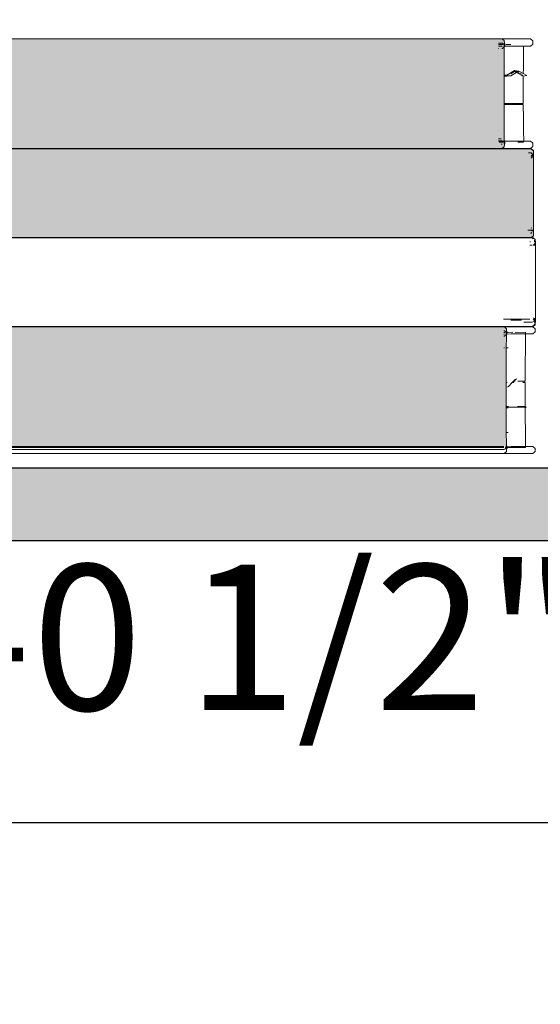
# Model space of a CAD drawing. Units: millimetres. Extents: x 7894 to 8038, y 6851 to 6951.
# Tile 18 of 49: x 7951.055 to 7954.632, y 6903.287 to 6910.053. Entities that reach past the tile are written whole.
import ezdxf

# ---------------------------------------------------------------- set-up
doc = ezdxf.new("R2010")
doc.units = ezdxf.units.MM
for name, color, linetype, lineweight in [('A-ANNO-DIMS', 2, 'Continuous', 18), ('A-FURN-BOOK', 8, 'Continuous', 13), ('A-FURN-SHLF', 7, 'Continuous', 30)]:
    doc.layers.add(name, color=color, linetype=linetype, lineweight=lineweight)
doc.layers.add('A-FURN-PATT', color=32, linetype='Continuous', lineweight=9, true_color=0xcd6928)
doc.styles.get("Standard").update_dxf_attribs({"font": 'arial.ttf'})
doc.dimstyles.new('ISO-25', dxfattribs={"dimtxt": 1, "dimasz": 1, "dimexe": 1.25, "dimexo": 0.625, "dimtad": 1, "dimdec": 0, "dimlunit": 4, "dimtxsty": 'Standard', "dimcen": 2.5, "dimclrt": 1, "dimadec": 0, "dimazin": 0, "dimtfac": 1, "dimtdec": 0, "dimtmove": 0, "dimatfit": 3, "dimfxl": 1, "dimarcsym": 0})

# ---------------------------------------------------------------- blocks, each defined once
blk = doc.blocks.new('*D23')
at = {"layer": 'A-ANNO-DIMS', "color": 0, "lineweight": -2, "transparency": 16777216}
for p, q in [((7940.0888, 6907.098), (7940.0888, 6947.7928)), ((7971.9356, 6928.989), (7971.9356, 6947.7928)), ((7941.0888, 6946.5428), (7970.9356, 6946.5428))]:
    blk.add_line(p, q, dxfattribs=at)
at = {"layer": 'A-ANNO-DIMS', "color": 0, "transparency": 16777216}
for points in [[(7941.0888, 6946.7095), (7941.0888, 6946.3762), (7940.0888, 6946.5428)], [(7970.9356, 6946.7095), (7970.9356, 6946.3762), (7971.9356, 6946.5428)]]:
    blk.add_solid(points, dxfattribs=at)
at = {"layer": 'Defpoints', "color": 0, "transparency": 16777216}
for p in [(7971.9356, 6946.5428), (7971.9356, 6928.364), (7940.0888, 6906.473)]:
    blk.add_point(p, dxfattribs=at)
at = {"layer": 'A-ANNO-DIMS', "color": 1, "transparency": 16777216, "insert": (7956.0122, 6947.6784), "char_height": 1, "attachment_point": 5}
blk.add_mtext('2\'-8"', dxfattribs=at)
blk = doc.blocks.new('*D24')
at = {"layer": 'A-ANNO-DIMS', "color": 0, "lineweight": -2, "transparency": 16777216}
for p, q in [((7953.3408, 6944.6059), (7936.9023, 6944.6059)), ((7938.1523, 6907.473), (7938.1523, 6943.6059)), ((7939.4638, 6906.473), (7936.9023, 6906.473))]:
    blk.add_line(p, q, dxfattribs=at)
at = {"layer": 'A-ANNO-DIMS', "color": 0, "transparency": 16777216}
for points in [[(7937.9856, 6943.6059), (7938.319, 6943.6059), (7938.1523, 6944.6059)], [(7937.9856, 6907.473), (7938.319, 6907.473), (7938.1523, 6906.473)]]:
    blk.add_solid(points, dxfattribs=at)
at = {"layer": 'Defpoints', "color": 0, "transparency": 16777216}
for p in [(7938.1523, 6944.6059), (7953.9658, 6944.6059), (7940.0888, 6906.473)]:
    blk.add_point(p, dxfattribs=at)
at = {"layer": 'A-ANNO-DIMS', "color": 1, "transparency": 16777216, "insert": (7937.0164, 6925.5395), "char_height": 1, "attachment_point": 5, "rotation": 90}
blk.add_mtext('3\'-2"', dxfattribs=at)
blk = doc.blocks.new('*D25')
at = {"layer": 'A-ANNO-DIMS', "color": 0, "lineweight": -2, "transparency": 16777216}
for p, q in [((7940.0888, 6905.848), (7940.0888, 6903.2865)), ((7964.3408, 6905.8484), (7964.3408, 6903.2865)), ((7941.0888, 6904.5365), (7963.3408, 6904.5365))]:
    blk.add_line(p, q, dxfattribs=at)
at = {"layer": 'A-ANNO-DIMS', "color": 0, "transparency": 16777216}
for points in [[(7941.0888, 6904.7032), (7941.0888, 6904.3699), (7940.0888, 6904.5365)], [(7963.3408, 6904.7032), (7963.3408, 6904.3699), (7964.3408, 6904.5365)]]:
    blk.add_solid(points, dxfattribs=at)
at = {"layer": 'Defpoints', "color": 0, "transparency": 16777216}
for p in [(7940.0888, 6906.473), (7964.3408, 6906.4734), (7964.3408, 6904.5365)]:
    blk.add_point(p, dxfattribs=at)
at = {"layer": 'A-ANNO-DIMS', "color": 1, "transparency": 16777216, "insert": (7952.2148, 6905.6786), "char_height": 1, "attachment_point": 5}
blk.add_mtext('2\'-0 1/2"', dxfattribs=at)
blk = doc.blocks.new('*D26')
at = {"layer": 'A-ANNO-DIMS', "color": 0, "lineweight": -2, "transparency": 16777216}
for p, q in [((7950.9654, 6918.7198), (7975.2272, 6918.7198)), ((7973.9772, 6917.7198), (7973.9772, 6907.4734)), ((7964.9658, 6906.4734), (7975.2272, 6906.4734))]:
    blk.add_line(p, q, dxfattribs=at)
at = {"layer": 'A-ANNO-DIMS', "color": 0, "transparency": 16777216}
for points in [[(7973.8105, 6917.7198), (7974.1439, 6917.7198), (7973.9772, 6918.7198)], [(7973.8105, 6907.4734), (7974.1439, 6907.4734), (7973.9772, 6906.4734)]]:
    blk.add_solid(points, dxfattribs=at)
at = {"layer": 'Defpoints', "color": 0, "transparency": 16777216}
for p in [(7950.3404, 6918.7198), (7964.3408, 6906.4734), (7973.9772, 6906.4734)]:
    blk.add_point(p, dxfattribs=at)
at = {"layer": 'A-ANNO-DIMS', "color": 1, "transparency": 16777216, "insert": (7972.8416, 6912.5966), "char_height": 1, "attachment_point": 5, "rotation": 90}
blk.add_mtext('1\'-0"', dxfattribs=at)

msp = doc.modelspace()

# ---------------------------------------------------------------- hatches: boundary and pattern name
at = {"layer": 'A-FURN-PATT'}
h = msp.add_hatch(color=256, dxfattribs=at)
h.dxf.hatch_style = 1
h.paths.add_polyline_path([(7942.8406, 6913.3629), (7942.8593, 6913.356), (7942.8677, 6913.356), (7942.8677, 6914.2132), (7942.876, 6914.2376), (7942.8813, 6914.2376), (7942.9022, 6914.2457), (7943.3657, 6914.2457), (7943.3844, 6914.2376), (7943.3861, 6914.2376), (7943.3858, 6914.2132), (7943.3852, 6913.2312), (7943.3944, 6906.9948), (7943.387, 6906.9732), (7943.4027, 6906.9732), (7943.403, 6906.9948), (7943.4029, 6908.4372), (7943.3944, 6914.2132), (7943.4169, 6914.2376), (7943.4198, 6914.2457), (7943.4555, 6914.2457), (7943.4603, 6914.238), (7943.8607, 6914.2452), (7943.8615, 6914.2457), (7943.8623, 6914.2452), (7943.8866, 6914.2457), (7943.8944, 6914.2402), (7943.9104, 6914.2376), (7943.9211, 6914.2132), (7943.9294, 6914.2376), (7943.9318, 6914.2376), (7943.9453, 6914.2398), (7943.9488, 6914.2457), (7943.9797, 6914.2452), (7943.9807, 6914.2457), (7943.9815, 6914.2451), (7944.3738, 6914.2376), (7944.3882, 6914.2457), (7944.4201, 6914.2457), (7944.4341, 6914.2376), (7944.4395, 6914.2376), (7944.4478, 6914.2132), (7944.4478, 6914.1031), (7944.4622, 6914.099), (7944.7359, 6914.1607), (7944.8923, 6914.2014), (7944.9541, 6914.2098), (7944.955, 6914.21), (7946.556, 6907.1325), (7946.5534, 6907.1122), (7946.5529, 6907.1152), (7946.499, 6907.103), (7946.3343, 6907.0604), (7946.0282, 6906.9914), (7945.6731, 6908.5712), (7944.4484, 6914.0015), (7944.4478, 6906.9948), (7944.4404, 6906.9732), (7947.0373, 6906.9734), (7964.3408, 6906.9734), (7964.3408, 6906.4734), (7947.0373, 6906.4734), (7940.0888, 6906.473), (7940.0888, 6906.973), (7941.9951, 6906.9731), (7941.9899, 6906.9898), (7941.9899, 6913.3353), (7941.9968, 6913.3574), (7942.003, 6913.3571), (7942.0169, 6913.3629), (7942.0366, 6913.3629), (7942.0378, 6913.3629), (7942.0479, 6913.356), (7942.8142, 6913.356), (7942.8157, 6913.356), (7942.8346, 6913.356)])
h.paths.add_polyline_path([(7942.8598, 6913.0201), (7942.861, 6913.3353), (7942.8677, 6906.9948), (7942.876, 6906.9759), (7942.876, 6906.9903), (7942.8813, 6914.2376), (7942.876, 6914.2321), (7942.876, 6914.2177), (7942.8809, 6906.9647), (7942.8784, 6906.9704), (7942.876, 6906.9704), (7942.8574, 6906.9704), (7942.8613, 6911.8549)], flags=16)
h.paths.add_polyline_path([(7942.8613, 6911.8549), (7942.8677, 6906.9948), (7942.8686, 6906.9921), (7942.8677, 6906.9898), (7942.8616, 6906.9704), (7942.8598, 6906.9704), (7942.8574, 6906.9704), (7942.0002, 6906.9704), (7941.9978, 6906.9704), (7941.996, 6906.9704), (7941.9899, 6906.9898), (7941.9978, 6906.9704), (7942.0002, 6906.9704), (7942.8598, 6906.9704), (7942.8616, 6906.9748)], flags=16)
h.paths.add_polyline_path([(7942.023, 6913.356), (7942.0169, 6913.3629), (7942.0366, 6913.3629), (7942.0378, 6913.3629), (7942.0367, 6913.3614), (7942.0369, 6913.356)], flags=16)
h.paths.add_polyline_path([(7942.0366, 6913.3629), (7942.0169, 6913.3629), (7942.0196, 6913.3598)], flags=0)
h.paths.add_polyline_path([(7942.0353, 6913.356), (7942.0369, 6913.356), (7942.0367, 6913.3614)], flags=0)
h.paths.add_polyline_path([(7943.9293, 6906.9759), (7943.9211, 6906.9948), (7943.9294, 6906.9704)], flags=0)
h.paths.add_polyline_path([(7943.9125, 6914.2132), (7943.8982, 6914.2376), (7943.8944, 6914.2402), (7943.8832, 6914.2421), (7943.8781, 6914.2367), (7943.8765, 6914.2376), (7943.8789, 6914.2376), (7943.8866, 6914.2457), (7943.8623, 6914.2452), (7943.8607, 6914.2452), (7943.8615, 6914.2457), (7943.8623, 6914.2452), (7943.8866, 6914.2457), (7943.8944, 6914.2402), (7943.8982, 6914.2376), (7943.9097, 6914.218), (7943.9125, 6914.2168), (7943.9079, 6906.9704), (7943.9104, 6906.9704), (7943.9211, 6914.2132), (7943.9294, 6914.2376), (7943.9318, 6914.2376), (7943.9453, 6914.2398), (7943.9488, 6914.2457), (7943.9797, 6914.2452), (7943.9807, 6914.2457), (7943.9815, 6914.2451), (7944.3738, 6914.2376), (7944.3882, 6914.2457), (7944.4201, 6914.2457), (7944.4341, 6914.2376), (7944.4395, 6914.2376), (7944.4395, 6914.2177), (7944.4341, 6914.0941), (7944.4478, 6914.1004), (7944.4513, 6914.1021), (7944.4622, 6914.099), (7944.4343, 6914.0927), (7944.429, 6914.0915), (7944.4341, 6914.069), (7944.4484, 6914.0015), (7944.4341, 6914.0649), (7944.4346, 6906.9704), (7944.4371, 6906.9704), (7944.4395, 6906.9759), (7944.4395, 6906.9704), (7943.931, 6906.9704), (7943.9128, 6906.9704), (7943.9079, 6906.9704)], flags=16)
h.paths.add_polyline_path([(7943.9211, 6914.2132), (7943.9294, 6914.2376), (7943.9318, 6914.2376), (7943.9453, 6914.2398), (7943.9488, 6914.2457), (7943.9797, 6914.2452), (7943.9807, 6914.2457), (7943.9815, 6914.2451), (7944.3738, 6914.2376), (7944.3882, 6914.2457), (7944.4201, 6914.2457), (7944.4321, 6914.2387), (7944.4249, 6914.2376), (7944.4041, 6914.2376), (7944.4032, 6914.2136), (7944.4032, 6914.2376), (7944.4025, 6914.2379), (7944.3897, 6914.2382), (7944.3753, 6914.2384), (7944.3738, 6914.2376), (7943.9815, 6914.2451), (7943.9488, 6914.2457), (7943.9453, 6914.2398), (7943.9294, 6914.2132), (7943.931, 6906.9721), (7943.931, 6906.9704), (7943.9294, 6906.9704), (7943.9293, 6906.9759), (7943.9294, 6914.2132), (7943.9439, 6914.2376), (7943.9318, 6914.2376)], flags=0)
h.paths.add_polyline_path([(7942.8813, 6914.2376), (7942.8778, 6914.2362), (7942.8796, 6914.2404), (7942.885, 6914.239)], flags=17)
h.paths.add_polyline_path([(7944.4116, 6914.242), (7944.4104, 6914.2408), (7944.4125, 6914.2418)], flags=0)
h.paths.add_polyline_path([(7944.3879, 6914.2382), (7944.3882, 6914.2457), (7944.4094, 6914.241), (7944.4103, 6914.2408), (7944.4036, 6914.2373), (7944.39, 6914.2447), (7944.3897, 6914.2382)], flags=0)
h.paths.add_polyline_path([(7963.1359, 6906.9526), (7963.1396, 6906.9526), (7963.1431, 6906.9582)], flags=16)
h.paths.add_polyline_path([(7954.3975, 6907.3902), (7954.397, 6907.3948), (7954.3984, 6907.4007), (7954.3975, 6907.567), (7954.3984, 6907.5978), (7954.3986, 6907.7694), (7954.3978, 6907.7989), (7954.399, 6907.8759), (7954.3992, 6907.9037), (7954.3944, 6907.9081), (7954.4019, 6907.9055), (7954.3996, 6907.93), (7954.3988, 6907.9307), (7954.3841, 6907.9429), (7946.6754, 6907.9429), (7946.6535, 6907.9232), (7946.6531, 6907.9127), (7946.6527, 6907.7694), (7946.6525, 6907.4007), (7946.653, 6907.1185), (7946.6574, 6907.1224), (7946.656, 6907.1145), (7946.6571, 6907.1135), (7946.6675, 6907.1209), (7946.7515, 6907.1209), (7946.9105, 6907.1209), (7954.3003, 6907.1209), (7954.3895, 6907.1209), (7954.3915, 6907.1191), (7954.3991, 6907.1209), (7954.399, 6907.1383), (7954.3978, 6907.2163), (7954.3986, 6907.2413)], flags=17)
h.paths.add_polyline_path([(7954.3003, 6907.1209), (7954.3003, 6907.1136), (7946.9105, 6907.1129), (7946.7516, 6907.1136), (7946.7515, 6907.1209), (7946.6675, 6907.1209), (7946.6531, 6907.1106), (7946.653, 6907.1185), (7946.6574, 6907.1224), (7946.656, 6907.1145), (7946.6571, 6907.1135), (7946.6675, 6907.1209), (7946.7515, 6907.1209), (7946.9105, 6907.1209)], flags=17)
h.paths.add_polyline_path([(7954.3981, 6907.9048), (7954.3944, 6907.9081), (7954.3997, 6907.9062), (7954.4007, 6907.9186), (7954.4019, 6907.9055), (7954.405, 6907.9072), (7954.4044, 6907.9046), (7954.4027, 6907.8974), (7954.4024, 6907.9009), (7954.3996, 6907.9034), (7954.3996, 6907.9025), (7954.3994, 6907.9023), (7954.3995, 6907.9035)], flags=17)
h = msp.add_hatch(color=256, dxfattribs=at)
h.dxf.hatch_style = 1
h.paths.add_polyline_path([(7954.384, 6909.6263), (7954.383, 6909.6719), (7954.3832, 6909.6719), (7954.3841, 6909.7804), (7954.3842, 6909.8528), (7954.3843, 6909.8691), (7954.3797, 6909.8762), (7954.3846, 6909.8799), (7954.3847, 6909.8812), (7954.3833, 6909.8825), (7954.3848, 6909.8826), (7954.3858, 6909.8967), (7954.3849, 6909.9082), (7954.384, 6909.909), (7954.384, 6909.9101), (7954.3682, 6909.9217), (7947.2251, 6909.9217), (7947.21, 6909.9101), (7947.2092, 6909.8906), (7947.2092, 6909.1993), (7947.2105, 6909.1985), (7947.2109, 6909.2125), (7947.2127, 6909.2113), (7947.2135, 6909.2114), (7947.2139, 6909.2117), (7947.2148, 6909.196), (7947.2105, 6909.1985), (7947.21, 6909.1798), (7947.2251, 6909.1682), (7947.2316, 6909.1682), (7954.3693, 6909.1682), (7954.384, 6909.1798), (7954.385, 6909.1814), (7954.3858, 6909.1921), (7954.3871, 6909.207), (7954.3814, 6909.2115), (7954.377, 6909.2116), (7954.3506, 6909.2116), (7954.3427, 6909.2213), (7954.373, 6909.2213), (7954.3747, 6909.2192), (7954.3833, 6909.2192), (7954.3833, 6909.2247), (7954.3843, 6909.2237), (7954.3842, 6909.2371), (7954.384, 6909.4541), (7954.3827, 6909.477), (7954.3832, 6909.477)])
h.paths.add_polyline_path([(7947.2139, 6909.8782), (7947.214, 6909.8795), (7947.2135, 6909.8785)], flags=16)
h.paths.add_polyline_path([(7947.2105, 6909.1985), (7947.2109, 6909.2125), (7947.2127, 6909.2113), (7947.2135, 6909.2114), (7947.2139, 6909.2117), (7947.2144, 6909.2034), (7947.2148, 6909.196)], flags=17)
h.paths.add_polyline_path([(7954.3858, 6909.1921), (7954.3848, 6909.2088), (7954.3871, 6909.207)], flags=17)
h.paths.add_polyline_path([(7954.5846, 6909.1237), (7954.5837, 6909.1245), (7954.5808, 6909.1271), (7954.5846, 6909.1307), (7954.5846, 6909.1519), (7954.5691, 6909.1658), (7946.8503, 6909.1658), (7946.8349, 6909.1546), (7946.8349, 6909.1307), (7946.8349, 6909.1147), (7946.8349, 6909.1147), (7946.8349, 6908.5685), (7946.8503, 6908.5572), (7954.5691, 6908.5572), (7954.5846, 6908.5685)])
h.paths.add_polyline_path([(7946.8375, 6909.1282), (7946.8349, 6909.1263), (7946.8349, 6909.1237), (7946.8473, 6909.1162), (7946.8503, 6909.1162)], flags=16)

# ---------------------------------------------------------------- linework, layer by layer
at = {"layer": 'A-FURN-BOOK'}
for p, q in [((7954.3693, 6909.9217), (7947.2251, 6909.9217)), ((7954.3721, 6909.8928), (7954.3445, 6909.8928)), ((7954.3463, 6909.8825), (7954.3445, 6909.883)), ((7954.3772, 6909.883), (7954.3463, 6909.8825)), ((7954.3756, 6909.9163), (7954.3693, 6909.9217)), ((7954.566, 6909.9217), (7954.3693, 6909.9217)), ((7954.3795, 6909.8859), (7954.3721, 6909.8928)), ((7954.3756, 6909.9163), (7954.384, 6909.9101)), ((7954.3833, 6909.8825), (7954.3848, 6909.8826)), ((7954.3848, 6909.8811), (7954.3833, 6909.8825)), ((7954.3848, 6909.8801), (7954.3833, 6909.8789)), ((7954.3833, 6909.8707), (7954.3848, 6909.8801)), ((7954.384, 6909.909), (7954.384, 6909.9101)), ((7954.3849, 6909.9082), (7954.384, 6909.909)), ((7954.3848, 6909.8826), (7954.3858, 6909.8967)), ((7954.3848, 6909.8826), (7954.3871, 6909.8832)), ((7954.3848, 6909.8811), (7954.3848, 6909.8826)), ((7954.3876, 6909.8785), (7954.3848, 6909.8811)), ((7954.3848, 6909.8801), (7954.3848, 6909.8811)), ((7954.3858, 6909.8967), (7954.3849, 6909.9082)), ((7954.3871, 6909.8832), (7954.3858, 6909.8967)), ((7954.3902, 6909.885), (7954.3871, 6909.8832)), ((7954.3871, 6909.8832), (7954.3897, 6909.8828)), ((7954.3876, 6909.8785), (7954.3871, 6909.8832)), ((7954.388, 6909.8698), (7954.3884, 6909.8735)), ((7954.3884, 6909.8735), (7954.3893, 6909.8811)), ((7954.3893, 6909.8811), (7954.3897, 6909.8828)), ((7954.3897, 6909.8828), (7954.3902, 6909.885)), ((7954.3897, 6909.8828), (7954.393, 6909.883)), ((7954.4013, 6909.8826), (7954.398, 6909.883)), ((7954.4298, 6909.883), (7954.4013, 6909.8826)), ((7954.566, 6909.9217), (7954.5815, 6909.9074)), ((7954.5815, 6909.885), (7954.566, 6909.8707)), ((7954.5815, 6909.9074), (7954.5815, 6909.885)), ((7954.3444, 6909.8707), (7954.3674, 6909.8707)), ((7954.3484, 6909.8549), (7954.3444, 6909.8549)), ((7954.3721, 6909.8549), (7954.3673, 6909.8549)), ((7954.3697, 6909.8686), (7954.3674, 6909.8686)), ((7954.3708, 6909.8694), (7954.3697, 6909.8686)), ((7954.3843, 6909.8661), (7954.3721, 6909.8549)), ((7954.3843, 6909.8691), (7954.3833, 6909.8707)), ((7954.3844, 6909.8707), (7954.3833, 6909.8707)), ((7954.3841, 6909.7804), (7954.3842, 6909.8528)), ((7954.3842, 6909.8528), (7954.3843, 6909.8661)), ((7954.3876, 6909.8692), (7954.3843, 6909.8661)), ((7954.3843, 6909.8661), (7954.3843, 6909.8691)), ((7954.388, 6909.8698), (7954.3844, 6909.8707)), ((7954.3876, 6909.8692), (7954.388, 6909.8698)), ((7954.388, 6909.8698), (7954.3935, 6909.8707)), ((7954.3935, 6909.8707), (7954.5169, 6909.8707)), ((7954.5169, 6909.8707), (7954.5162, 6909.8039)), ((7954.5169, 6909.8707), (7954.566, 6909.8707)), ((7954.3456, 6909.8039), (7954.3444, 6909.8039)), ((7954.3832, 6909.673), (7954.3841, 6909.7804)), ((7954.5162, 6909.8039), (7954.5157, 6909.7171)), ((7954.384, 6909.672), (7954.3832, 6909.673)), ((7954.3832, 6909.672), (7954.3832, 6909.673)), ((7954.3832, 6909.672), (7954.384, 6909.672)), ((7954.3832, 6909.6692), (7954.3832, 6909.672)), ((7954.3988, 6909.673), (7954.384, 6909.672)), ((7954.3988, 6909.673), (7954.3999, 6909.6721)), ((7954.3999, 6909.6721), (7954.4015, 6909.673)), ((7954.4027, 6909.673), (7954.4015, 6909.673)), ((7954.4027, 6909.673), (7954.4549, 6909.7037)), ((7954.4548, 6909.6961), (7954.4302, 6909.6819)), ((7954.4308, 6909.6683), (7954.4678, 6909.6896)), ((7954.467, 6909.6976), (7954.4548, 6909.6961)), ((7954.4623, 6909.6923), (7954.4548, 6909.6961)), ((7954.4857, 6909.6999), (7954.4549, 6909.7037)), ((7954.4549, 6909.7037), (7954.467, 6909.6976)), ((7954.4857, 6909.6999), (7954.467, 6909.6976)), ((7954.467, 6909.6976), (7954.4715, 6909.6953)), ((7954.4678, 6909.6896), (7954.4748, 6909.6936)), ((7954.5005, 6909.673), (7954.4678, 6909.6896)), ((7954.4748, 6909.6936), (7954.4857, 6909.6999)), ((7954.4748, 6909.6936), (7954.5038, 6909.6789)), ((7954.5156, 6909.6831), (7954.4857, 6909.6999)), ((7954.509, 6909.673), (7954.5005, 6909.673)), ((7954.508, 6909.6692), (7954.5005, 6909.673)), ((7954.5157, 6909.7171), (7954.5156, 6909.6831)), ((7954.5401, 6909.6692), (7954.5156, 6909.6831)), ((7954.3832, 6909.6692), (7954.384, 6909.6692)), ((7954.3832, 6909.6679), (7954.3832, 6909.6692)), ((7954.3832, 6909.6679), (7954.4062, 6909.6681)), ((7954.3832, 6909.6654), (7954.3832, 6909.6679)), ((7954.3832, 6909.6654), (7954.384, 6909.6654)), ((7954.384, 6909.6654), (7954.3832, 6909.6643)), ((7954.3832, 6909.6643), (7954.3832, 6909.6654)), ((7954.384, 6909.6263), (7954.3832, 6909.6643)), ((7954.3832, 6909.477), (7954.384, 6909.6263)), ((7954.384, 6909.6692), (7954.4062, 6909.6681)), ((7954.3999, 6909.6645), (7954.384, 6909.6654)), ((7954.4016, 6909.6654), (7954.3999, 6909.6645)), ((7954.4308, 6909.6683), (7954.4016, 6909.6654)), ((7954.4062, 6909.6681), (7954.4016, 6909.6654)), ((7954.4062, 6909.6681), (7954.4072, 6909.6692)), ((7954.4308, 6909.6683), (7954.4072, 6909.6692)), ((7954.508, 6909.6692), (7954.5122, 6909.6692)), ((7954.5155, 6909.6654), (7954.508, 6909.6692)), ((7954.5155, 6909.6654), (7954.5154, 6909.6214)), ((7954.5154, 6909.477), (7954.5154, 6909.6214)), ((7954.5401, 6909.6692), (7954.5155, 6909.6654)), ((7954.3832, 6909.477), (7954.384, 6909.477)), ((7954.3832, 6909.4694), (7954.3832, 6909.477)), ((7954.3832, 6909.4694), (7954.3998, 6909.4695)), ((7954.384, 6909.4541), (7954.3832, 6909.4694)), ((7954.384, 6909.477), (7954.3998, 6909.4771)), ((7954.3998, 6909.4771), (7954.5154, 6909.477)), ((7954.3998, 6909.4695), (7954.5154, 6909.4694)), ((7954.5154, 6909.477), (7954.4662, 6909.4732)), ((7954.4662, 6909.4732), (7954.5154, 6909.4694)), ((7954.5157, 6909.3775), (7954.5154, 6909.4694)), ((7954.384, 6909.4541), (7954.3842, 6909.2371)), ((7954.5157, 6909.3775), (7954.5162, 6909.2907)), ((7954.3444, 6909.2907), (7954.3456, 6909.2907)), ((7954.5162, 6909.2907), (7954.518, 6909.2192)), ((7954.3633, 6909.235), (7954.3444, 6909.235)), ((7954.3677, 6909.2213), (7954.3444, 6909.2213)), ((7954.3444, 6909.2192), (7954.3725, 6909.2192)), ((7954.3501, 6909.2121), (7954.377, 6909.2116)), ((7954.377, 6909.2116), (7954.3506, 6909.2116)), ((7954.3704, 6909.1971), (7954.3622, 6909.1971)), ((7954.3725, 6909.2192), (7954.3708, 6909.2205)), ((7954.3747, 6909.2192), (7954.3725, 6909.2192)), ((7954.3747, 6909.2192), (7954.3788, 6909.2154)), ((7954.3784, 6909.2147), (7954.3747, 6909.2192)), ((7954.3805, 6909.2192), (7954.3747, 6909.2192)), ((7954.3843, 6909.2237), (7954.3828, 6909.2251)), ((7954.3833, 6909.2192), (7954.3843, 6909.2207)), ((7954.3844, 6909.2192), (7954.3833, 6909.2192)), ((7954.3833, 6909.212), (7954.3833, 6909.2192)), ((7954.3833, 6909.212), (7954.3847, 6909.2118)), ((7954.3847, 6909.2118), (7954.3833, 6909.2113)), ((7954.3848, 6909.2098), (7954.3833, 6909.2113)), ((7954.3848, 6909.2088), (7954.3833, 6909.2074)), ((7954.3843, 6909.2237), (7954.3842, 6909.2371)), ((7954.3843, 6909.2207), (7954.3843, 6909.2237)), ((7954.3876, 6909.2207), (7954.3843, 6909.2237)), ((7954.388, 6909.2201), (7954.3844, 6909.2192)), ((7954.3876, 6909.2114), (7954.3847, 6909.2118)), ((7954.3848, 6909.2098), (7954.3847, 6909.2118)), ((7954.3876, 6909.2114), (7954.3848, 6909.2098)), ((7954.3848, 6909.2098), (7954.3848, 6909.2088)), ((7954.3848, 6909.2088), (7954.3858, 6909.1921)), ((7954.3848, 6909.2088), (7954.3871, 6909.207)), ((7954.3858, 6909.1921), (7954.3871, 6909.207)), ((7954.3871, 6909.207), (7954.3876, 6909.2114)), ((7954.3871, 6909.207), (7954.3902, 6909.2049)), ((7954.388, 6909.2201), (7954.3876, 6909.2207)), ((7954.3935, 6909.2192), (7954.388, 6909.2201)), ((7954.3884, 6909.2161), (7954.388, 6909.2201)), ((7954.3893, 6909.2088), (7954.3884, 6909.2161)), ((7954.3902, 6909.2049), (7954.3893, 6909.2088)), ((7954.518, 6909.2192), (7954.3935, 6909.2192)), ((7954.4778, 6909.2117), (7954.4788, 6909.2116)), ((7954.517, 6909.2116), (7954.4788, 6909.2116)), ((7954.518, 6909.2192), (7954.517, 6909.2116)), ((7954.518, 6909.2192), (7954.566, 6909.2192)), ((7954.566, 6909.2192), (7954.5815, 6909.2049)), ((7954.5815, 6909.2049), (7954.5815, 6909.1825)), ((7954.5691, 6909.1658), (7946.8503, 6909.1658)), ((7947.2316, 6909.1682), (7954.3693, 6909.1682)), ((7954.3693, 6909.1682), (7954.384, 6909.1798)), ((7954.3693, 6909.1682), (7954.566, 6909.1682)), ((7954.384, 6909.1798), (7954.385, 6909.1814)), ((7954.385, 6909.1814), (7954.3858, 6909.1921)), ((7954.5691, 6909.1377), (7954.5514, 6909.1377)), ((7954.5815, 6909.1825), (7954.566, 6909.1682)), ((7954.5691, 6909.1658), (7954.5846, 6909.1519)), ((7954.5846, 6909.1528), (7954.5691, 6909.1658)), ((7954.5691, 6909.1658), (7954.5846, 6909.1546)), ((7954.5808, 6909.1271), (7954.5691, 6909.1377)), ((7954.5846, 6909.1307), (7954.5808, 6909.1271)), ((7954.5846, 6909.1528), (7954.5846, 6909.1546)), ((7954.5846, 6909.1519), (7954.5846, 6909.1528)), ((7954.5846, 6909.1307), (7954.5846, 6909.1519)), ((7954.5846, 6909.1263), (7954.5846, 6909.1307)), ((7954.5808, 6909.1271), (7954.5691, 6909.1162)), ((7954.5837, 6909.1245), (7954.5691, 6909.1141)), ((7954.5846, 6909.1147), (7954.5691, 6909.1008)), ((7954.5837, 6909.1245), (7954.5808, 6909.1271)), ((7954.5837, 6909.1245), (7954.5846, 6909.1263)), ((7954.5846, 6909.1252), (7954.5837, 6909.1245)), ((7954.5846, 6909.1237), (7954.5837, 6909.1245)), ((7954.5846, 6909.1263), (7954.5846, 6909.1252)), ((7954.5846, 6909.1252), (7954.5846, 6909.1237)), ((7954.5846, 6909.1244), (7954.5846, 6909.1252)), ((7954.5846, 6909.1237), (7954.5846, 6909.1244)), ((7954.5846, 6909.1147), (7954.5846, 6909.1237)), ((7954.5846, 6909.1147), (7954.5846, 6908.5685)), ((7954.5462, 6908.6068), (7954.5691, 6908.6068)), ((7954.5717, 6908.6199), (7954.5691, 6908.6222)), ((7954.5691, 6908.6068), (7954.5781, 6908.5987)), ((7954.574, 6908.5898), (7954.5691, 6908.5853)), ((7954.5794, 6908.6014), (7954.571, 6908.6075)), ((7954.5831, 6908.6096), (7954.5811, 6908.6114)), ((7954.5691, 6908.5572), (7946.8503, 6908.5572)), ((7947.3682, 6908.5542), (7954.5763, 6908.5542)), ((7954.5659, 6908.5261), (7954.5608, 6908.5261)), ((7954.5691, 6908.5853), (7954.5639, 6908.5853)), ((7954.5846, 6908.5685), (7954.5691, 6908.5572)), ((7954.5763, 6908.5542), (7954.583, 6908.5482)), ((7954.5828, 6908.5542), (7954.5763, 6908.5542)), ((7954.5828, 6908.5542), (7954.5979, 6908.543)), ((7954.592, 6908.5386), (7954.5926, 6908.5341)), ((7954.5926, 6908.5341), (7954.593, 6908.5271)), ((7954.5966, 6908.5136), (7954.5973, 6908.5223)), ((7954.5974, 6908.5247), (7954.5979, 6908.543)), ((7954.5979, 6908.543), (7954.5987, 6908.524)), ((7954.5987, 6908.524), (7954.599, 6908.4287)), ((7954.5763, 6908.5046), (7954.5609, 6908.5046)), ((7954.5853, 6908.504), (7954.5841, 6908.5045)), ((7954.5853, 6908.504), (7954.5944, 6908.5122)), ((7954.5939, 6908.5132), (7954.5916, 6908.5147)), ((7954.5944, 6908.5031), (7954.5923, 6908.5013)), ((7954.5936, 6908.5175), (7954.5939, 6908.5132)), ((7954.5939, 6908.5132), (7954.5944, 6908.5122)), ((7954.5944, 6908.5122), (7954.596, 6908.5121)), ((7954.5948, 6908.5056), (7954.5944, 6908.5031)), ((7954.596, 6908.5121), (7954.5948, 6908.5056)), ((7954.5966, 6908.5136), (7954.596, 6908.5121)), ((7954.599, 6908.4287), (7954.5992, 6908.3136)), ((7954.5992, 6908.3136), (7954.5992, 6908.1815)), ((7954.5992, 6908.1815), (7954.5988, 6908.0011)), ((7954.5005, 6907.9952), (7954.38, 6907.9952)), ((7954.5005, 6907.988), (7954.4292, 6907.9877)), ((7954.5005, 6907.9952), (7954.5005, 6907.988)), ((7954.5609, 6907.9952), (7954.5005, 6907.9952)), ((7954.5944, 6907.9876), (7954.5837, 6907.9956)), ((7954.5939, 6907.9867), (7954.5837, 6907.9781)), ((7954.5944, 6907.9967), (7954.5856, 6908.0046)), ((7954.5935, 6907.9799), (7954.5931, 6907.9727)), ((7954.5939, 6907.9867), (7954.5935, 6907.9799)), ((7954.5944, 6907.9876), (7954.5939, 6907.9867)), ((7954.5944, 6907.9967), (7954.5948, 6907.9942)), ((7954.5965, 6907.9873), (7954.5944, 6907.9876)), ((7954.5948, 6907.9942), (7954.5959, 6907.9889)), ((7954.5959, 6907.9889), (7954.5965, 6907.9873)), ((7954.5965, 6907.9873), (7954.5971, 6907.9861)), ((7954.5971, 6907.9861), (7954.5974, 6907.9751)), ((7954.5988, 6908.0011), (7954.5987, 6907.9759)), ((7946.6754, 6907.9429), (7954.3841, 6907.9429)), ((7954.5828, 6907.9456), (7947.3682, 6907.9456)), ((7954.3869, 6907.9148), (7954.3822, 6907.9148)), ((7954.3904, 6907.9377), (7954.3841, 6907.9429)), ((7954.3841, 6907.9429), (7954.5808, 6907.9429)), ((7954.3943, 6907.9081), (7954.3869, 6907.9148)), ((7954.3981, 6907.9312), (7954.3904, 6907.9377)), ((7954.3904, 6907.9377), (7954.3988, 6907.9317)), ((7954.3998, 6907.9298), (7954.3988, 6907.9317)), ((7954.3998, 6907.9298), (7954.3988, 6907.9307)), ((7954.3996, 6907.9047), (7954.4007, 6907.9186)), ((7954.4007, 6907.9186), (7954.3998, 6907.9298)), ((7954.4019, 6907.9055), (7954.4007, 6907.9186)), ((7954.5785, 6907.9737), (7954.5198, 6907.9737)), ((7954.583, 6907.9517), (7954.5797, 6907.9487)), ((7954.5808, 6907.9429), (7954.5963, 6907.929)), ((7954.5979, 6907.9569), (7954.5828, 6907.9456)), ((7954.5917, 6907.9595), (7954.5886, 6907.9567)), ((7954.5924, 6907.9639), (7954.5917, 6907.9595)), ((7954.5963, 6907.929), (7954.5963, 6907.9072)), ((7954.5987, 6907.9759), (7954.5974, 6907.9751)), ((7954.5979, 6907.9569), (7954.5974, 6907.9751)), ((7954.3911, 6907.9043), (7954.3821, 6907.9042)), ((7954.3845, 6907.8912), (7954.3821, 6907.8912)), ((7954.3869, 6907.8779), (7954.3821, 6907.8779)), ((7954.3856, 6907.892), (7954.3845, 6907.8912)), ((7954.3991, 6907.8889), (7954.3869, 6907.8779)), ((7954.3978, 6907.7989), (7954.399, 6907.8759)), ((7954.398, 6907.8933), (7954.3996, 6907.9025)), ((7954.3991, 6907.8918), (7954.398, 6907.8933)), ((7954.3992, 6907.8933), (7954.398, 6907.8933)), ((7954.3996, 6907.9047), (7954.3981, 6907.9048)), ((7954.3996, 6907.9034), (7954.3981, 6907.9048)), ((7954.3996, 6907.9025), (7954.3981, 6907.9013)), ((7954.399, 6907.8759), (7954.3991, 6907.8889)), ((7954.3991, 6907.8889), (7954.3991, 6907.8918)), ((7954.4024, 6907.8918), (7954.3991, 6907.8889)), ((7954.4028, 6907.8925), (7954.3992, 6907.8933)), ((7954.4019, 6907.9055), (7954.3996, 6907.9047)), ((7954.3996, 6907.9034), (7954.3996, 6907.9047)), ((7954.3996, 6907.9025), (7954.3996, 6907.9034)), ((7954.4024, 6907.9009), (7954.3996, 6907.9025)), ((7954.405, 6907.9072), (7954.4019, 6907.9055)), ((7954.4044, 6907.9046), (7954.4019, 6907.9055)), ((7954.4024, 6907.9009), (7954.4019, 6907.9055)), ((7954.4024, 6907.8918), (7954.4028, 6907.8925)), ((7954.4028, 6907.8925), (7954.4032, 6907.8961)), ((7954.4312, 6907.8933), (7954.4028, 6907.8925)), ((7954.4032, 6907.8961), (7954.4041, 6907.9034)), ((7954.4041, 6907.9034), (7954.4044, 6907.9046)), ((7954.4044, 6907.9046), (7954.405, 6907.9072)), ((7954.4147, 6907.9044), (7954.4044, 6907.9046)), ((7954.4439, 6907.9047), (7954.4147, 6907.9044)), ((7954.5303, 6907.8933), (7954.4312, 6907.8933)), ((7954.4621, 6907.9047), (7954.4633, 6907.9045)), ((7954.5304, 6907.9047), (7954.4633, 6907.9045)), ((7954.5303, 6907.8933), (7954.5296, 6907.7989)), ((7954.5304, 6907.9047), (7954.5303, 6907.8933)), ((7954.5303, 6907.8933), (7954.5808, 6907.8933)), ((7954.5963, 6907.9072), (7954.5808, 6907.8933)), ((7954.3858, 6907.7989), (7954.3818, 6907.7989)), ((7954.3986, 6907.7694), (7954.3978, 6907.7989)), ((7954.4125, 6907.7989), (7954.3978, 6907.7989)), ((7954.5296, 6907.7989), (7954.5291, 6907.687)), ((7954.3984, 6907.5978), (7954.3986, 6907.7694)), ((7954.5288, 6907.5685), (7954.5291, 6907.687)), ((7954.3975, 6907.5685), (7954.3984, 6907.5978)), ((7954.4482, 6907.5685), (7954.4601, 6907.5807)), ((7954.4681, 6907.5856), (7954.4503, 6907.5685)), ((7954.4681, 6907.5856), (7954.4601, 6907.5807)), ((7954.3975, 6907.5587), (7954.3975, 6907.5685)), ((7954.3975, 6907.5685), (7954.4011, 6907.5685)), ((7954.3984, 6907.4007), (7954.3975, 6907.5587)), ((7954.4049, 6907.5587), (7954.3975, 6907.5587)), ((7954.4079, 6907.5271), (7954.4132, 6907.532)), ((7954.4386, 6907.5587), (7954.4132, 6907.532)), ((7954.4386, 6907.5587), (7954.4352, 6907.5587)), ((7954.4503, 6907.5685), (7954.4386, 6907.5587)), ((7954.4386, 6907.5587), (7954.4482, 6907.5685)), ((7954.4505, 6907.5587), (7954.4424, 6907.5587)), ((7954.4452, 6907.5685), (7954.4482, 6907.5685)), ((7954.4503, 6907.5685), (7954.4606, 6907.5685)), ((7954.4555, 6907.5587), (7954.4542, 6907.5587)), ((7954.4771, 6907.5685), (7954.5288, 6907.5685)), ((7954.5288, 6907.5587), (7954.5118, 6907.5587)), ((7954.5288, 6907.5685), (7954.5181, 6907.5636)), ((7954.5181, 6907.5636), (7954.5288, 6907.5587)), ((7954.5288, 6907.4516), (7954.5288, 6907.5587)), ((7954.5288, 6907.4516), (7954.5289, 6907.3948)), ((7954.397, 6907.3948), (7954.3984, 6907.4007)), ((7954.3975, 6907.39), (7954.397, 6907.3948)), ((7954.4133, 6907.3948), (7954.397, 6907.3948)), ((7954.3976, 6907.3851), (7954.3975, 6907.39)), ((7954.5358, 6907.39), (7954.3975, 6907.39)), ((7954.3986, 6907.2413), (7954.3976, 6907.3851)), ((7954.3976, 6907.3851), (7954.4122, 6907.3851)), ((7954.5289, 6907.3948), (7954.4758, 6907.3948)), ((7954.5289, 6907.3948), (7954.5358, 6907.39)), ((7954.5289, 6907.3851), (7954.5358, 6907.39)), ((7954.5291, 6907.3283), (7954.5289, 6907.3851)), ((7954.5291, 6907.3283), (7954.5296, 6907.2163)), ((7954.3978, 6907.2163), (7954.3986, 6907.2413)), ((7954.399, 6907.1383), (7954.3978, 6907.2163)), ((7954.3978, 6907.2163), (7954.4125, 6907.2163)), ((7954.5296, 6907.2163), (7954.5303, 6907.1209)), ((7954.3822, 6907.0994), (7946.6728, 6907.0994)), ((7954.3003, 6907.1209), (7946.9105, 6907.1209)), ((7954.3003, 6907.1136), (7946.9105, 6907.1129)), ((7954.3003, 6907.1209), (7954.3003, 6907.1136)), ((7954.3821, 6907.1209), (7954.3003, 6907.1209)), ((7954.3003, 6907.1136), (7954.3597, 6907.1134)), ((7954.3597, 6907.1134), (7954.3821, 6907.1129)), ((7954.3869, 6907.0994), (7954.3852, 6907.0994)), ((7954.3996, 6907.1117), (7954.3869, 6907.0994)), ((7954.3915, 6907.1129), (7954.3984, 6907.1129)), ((7954.3984, 6907.1129), (7954.3932, 6907.1165)), ((7954.3936, 6907.1173), (7954.3984, 6907.1129)), ((7954.3992, 6907.1209), (7954.3953, 6907.1209)), ((7954.3991, 6907.1253), (7954.3979, 6907.1264)), ((7954.3984, 6907.1129), (7954.3992, 6907.1209)), ((7954.3996, 6907.1117), (7954.3984, 6907.1129)), ((7954.3991, 6907.1253), (7954.399, 6907.1383)), ((7954.3991, 6907.1224), (7954.3991, 6907.1253)), ((7954.4024, 6907.1224), (7954.3991, 6907.1253)), ((7954.3992, 6907.1209), (7954.3991, 6907.1224)), ((7954.4028, 6907.1217), (7954.3992, 6907.1209)), ((7954.4024, 6907.1133), (7954.3996, 6907.1117)), ((7954.3996, 6907.1117), (7954.3996, 6907.1108)), ((7954.3996, 6907.1117), (7954.4019, 6907.109)), ((7954.4041, 6907.1108), (7954.3996, 6907.1117)), ((7954.3996, 6907.1108), (7954.4006, 6907.0945)), ((7954.4006, 6907.0945), (7954.4019, 6907.109)), ((7954.4019, 6907.109), (7954.4024, 6907.1133)), ((7954.4019, 6907.109), (7954.405, 6907.107)), ((7954.4028, 6907.1217), (7954.4024, 6907.1224)), ((7954.4024, 6907.1133), (7954.4038, 6907.1129)), ((7954.4312, 6907.1209), (7954.4028, 6907.1217)), ((7954.4032, 6907.1179), (7954.4028, 6907.1217)), ((7954.4038, 6907.1129), (7954.4032, 6907.1179)), ((7954.4038, 6907.1129), (7954.4147, 6907.1133)), ((7954.4041, 6907.1108), (7954.4038, 6907.1129)), ((7954.4696, 6907.1131), (7954.4041, 6907.1108)), ((7954.405, 6907.107), (7954.4041, 6907.1108)), ((7954.4147, 6907.1133), (7954.4696, 6907.1131)), ((7954.4312, 6907.1209), (7954.5303, 6907.1209)), ((7954.4696, 6907.1131), (7954.5304, 6907.1129)), ((7954.5303, 6907.1209), (7954.5304, 6907.1129)), ((7954.5303, 6907.1209), (7954.5808, 6907.1209)), ((7954.5808, 6907.1209), (7954.5963, 6907.107)), ((7954.5963, 6907.107), (7954.5963, 6907.0852)), ((7954.3841, 6907.0713), (7946.669, 6907.0713)), ((7954.3841, 6907.0713), (7954.3988, 6907.0825)), ((7954.3841, 6907.0713), (7954.5808, 6907.0713)), ((7954.3988, 6907.0825), (7954.3998, 6907.0841)), ((7954.3998, 6907.0841), (7954.4006, 6907.0945)), ((7954.5963, 6907.0852), (7954.5808, 6907.0713))]:
    msp.add_line(p, q, dxfattribs=at)
at = {"layer": 'A-FURN-SHLF'}
for p, q in [((7947.0373, 6906.9734), (7964.3408, 6906.9734)), ((7947.0373, 6906.4734), (7964.3408, 6906.4734))]:
    msp.add_line(p, q, dxfattribs=at)

# ---------------------------------------------------------------- dimensions: what is measured, and where the dimension line sits
at = {"layer": 'A-ANNO-DIMS'}
for base, p2, picture, middle in [((7971.9356, 6946.5428), (7971.9356, 6928.364), '*D23', (7956.0122, 6947.6784)), ((7964.3408, 6904.5365), (7964.3408, 6906.4734), '*D25', (7952.2148, 6905.6786))]:
    dim = msp.add_linear_dim(base=base, p1=(7940.0888, 6906.473), p2=p2, dimstyle='ISO-25', override={"dimdec": 1, "dimlfac": 1, "dimrnd": 0, "dimzin": 1, "dimdsep": 46, "dimlunit": 4, "dimfrac": 2}, dxfattribs=at)
    dim.commit()
    dim.dimension.update_dxf_attribs({"geometry": picture, "text_midpoint": middle})
for base, p1, p2, picture, middle in [((7938.1523, 6944.6059), (7940.0888, 6906.473), (7953.9658, 6944.6059), '*D24', (7937.0164, 6925.5395)), ((7973.9772, 6906.4734), (7950.3404, 6918.7198), (7964.3408, 6906.4734), '*D26', (7972.8416, 6912.5966))]:
    dim = msp.add_linear_dim(base=base, p1=p1, p2=p2, angle=90, dimstyle='ISO-25', override={"dimdec": 1, "dimlfac": 1, "dimrnd": 0, "dimzin": 1, "dimdsep": 46, "dimlunit": 4, "dimfrac": 2}, dxfattribs=at)
    dim.commit()
    dim.dimension.update_dxf_attribs({"geometry": picture, "text_midpoint": middle})

doc.saveas('drawing.dxf')
